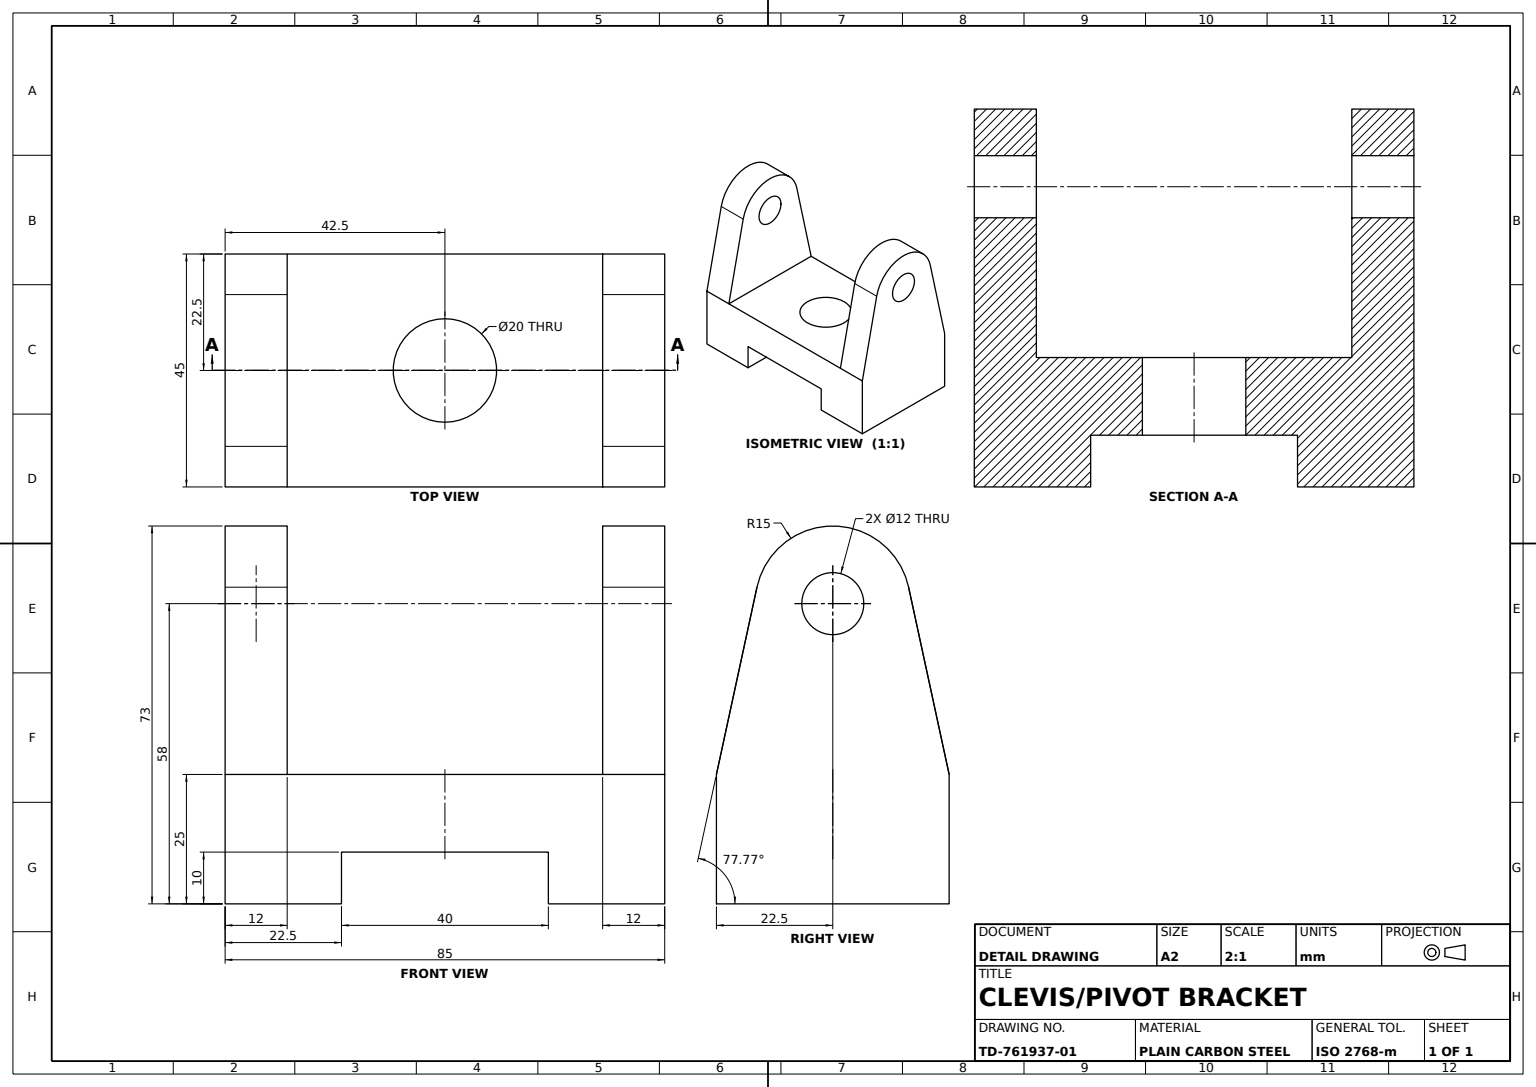
SolidWorks part; units mm, degrees
material "Plain Carbon Steel"
ref_plane "Front Plane" through (0, 0, 0) normal (0, 0, 1) x (1, 0, 0)
ref_plane "Top Plane" through (0, 0, 0) normal (0, 1, 0) x (1, 0, 0)
ref_plane "Right Plane" through (0, 0, 0) normal (1, 0, 0) x (0, 0, -1)
sketch "T-Slot Base Profile" plane through (0, 0, 0) normal (0, 0, 1) x (1, 0, 0)
  line L1 (-20, 0) -> (-42.5, 0)
  line L2 (-42.5, 0) -> (-42.5, 25)
  line L3 (-42.5, 25) -> (42.5, 25)
  line L4 (42.5, 25) -> (42.5, 0)
  line L5 (42.5, 0) -> (20, 0)
  line L6 (20, 0) -> (20, 10)
  line L7 (20, 10) -> (-20, 10)
  line L8 (-20, 10) -> (-20, 0)
  point P4 (0, 0)
  dimension "D1" = 40
  dimension "D2" = 22.5
  dimension "D3" = 22.5
  dimension "D4" = 25
  dimension "D5" = 10
  dimension "D6" = 25
  dimension "D7" = 42.5
extrude "T-Slot Base" add sketch "T-Slot Base Profile" along normal blind 45
sketch "Centre Bore Sketch" plane through (0, 25, 0) normal (0, 1, 0) x (1, 0, 0)
  line L0 (42.5, 0) -> (-42.5, 0) construction
  line L1 (42.5, -45) -> (42.5, 0) construction
  circle A0 centre (0, -22.5) radius 10
  dimension "D1" = 20
  dimension "D2" = 22.5
  dimension "D3" = 42.5
extrude "Centre Bore Ø20" cut sketch "Centre Bore Sketch" against normal blind 45
sketch "Clevis Lug 1 Profile" plane through (-42.5, 0, 0) normal (-1, 0, 0) x (0, 0, 1)
  line L0 (45, 0) -> (0, 0) construction
  line L1 (45, 25) -> (45, 0) construction
  line L2 (0, 25) -> (45, 25)
  line L3 (45, 25) -> (37.1597, 61.1771)
  line L4 (0, 25) -> (7.8403, 61.1771)
  arc A0 (37.1597, 61.1771) -> (7.8403, 61.1771) centre (22.5, 58) ccw
  circle A1 centre (22.5, 58) radius 6
  dimension "D1" = 30
  dimension "D2" = 12
  dimension "D3" = 58
  dimension "D4" = 22.5
extrude "Clevis Lug 1" add sketch "Clevis Lug 1 Profile" against normal blind 12
sketch "Clevis Lug 2 Profile" plane through (42.5, 0, 0) normal (1, 0, 0) x (0, 0, -1)
  line L0 (-37.1597, 61.1771) -> (-45, 25)
  line L1 (-45, 25) -> (0, 25)
  line L2 (0, 25) -> (-7.8403, 61.1771)
  circle A0 centre (-22.5, 58) radius 6
  arc A1 (-7.8403, 61.1771) -> (-37.1597, 61.1771) centre (-22.5, 58) ccw
  dimension "D2" = 12
extrude "Clevis Lug 2" add sketch "Clevis Lug 2 Profile" against normal blind 12
